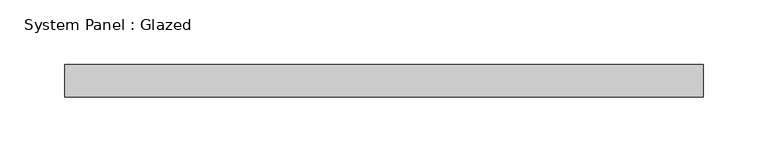
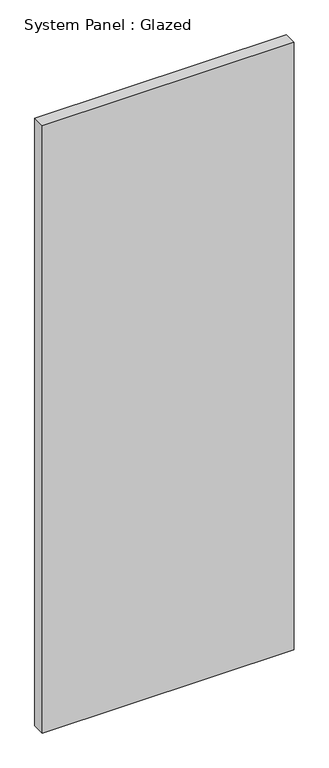
"""IFC4 building model written with IfcOpenShell, lengths in millimetres: plate geometry, System Panel : Glazed."""

from ifc_helpers import new_model, si_unit, origin, origin_with_axes, place, context, project, spatial, polyline, outline, extrude, source, transform, mapped, element, save


def system_panel_glazed_71b5d3b3(model_context):
    return source(origin(), model_context, "Body", "SweptSolid", [
        extrude(outline(polyline([(247.65, 19.05), (-247.65, 19.05), (-247.65, 44.45), (247.65, 44.45), (247.65, 19.05)])), origin_with_axes(), (0.0, 0.0, 1.0), 1261.8321364),
    ])


if __name__ == "__main__":
    model = new_model("IFC4")
    model_context = context("Model", 3, world=origin())
    ifc_project = project(units=[si_unit("LENGTHUNIT", "METRE", prefix="MILLI")], contexts=[model_context])
    site = spatial("IfcSite", under=ifc_project)
    building = spatial("IfcBuilding", under=site)
    placement = place(None, origin())
    system_panel_glazed_shape = system_panel_glazed_71b5d3b3(model_context)
    element("IfcPlate", 1, ObjectType="System Panel : Glazed", at=placement, inside=building, context=model_context, shape_type="MappedRepresentation", body=[
        mapped(system_panel_glazed_shape, transform((0.0, 0.0, 0.0), x_axis=(1.0, 0.0, 0.0), y_axis=(0.0, 1.0, 0.0), z_axis=(0.0, 0.0, 1.0))),
    ])
    save(model, "model.ifc")

# Revit data of these elements
# Type "System Panel : Glazed"
#   Construction Type Id = "GSP4R"
#   Analytic Construction = "1/8 in Pilkington single glazing"
#   Visual Light Transmittance = 0.9
#   Solar Heat Gain Coefficient = 0.86
#   Heat Transfer Coefficient (U) = 1.18115 BTU/(h·ft²·°F)
#   Define Thermal Properties by = 1
# Element 1 (IfcPlate, "System Panel : Glazed")
#   Materials on its faces: "Glass"
# Materials
#   "Glass": class "Glass", colour RGB 0 128 192, transparency 0.75, Description = "Soda Lime Glass", Cost = 0
